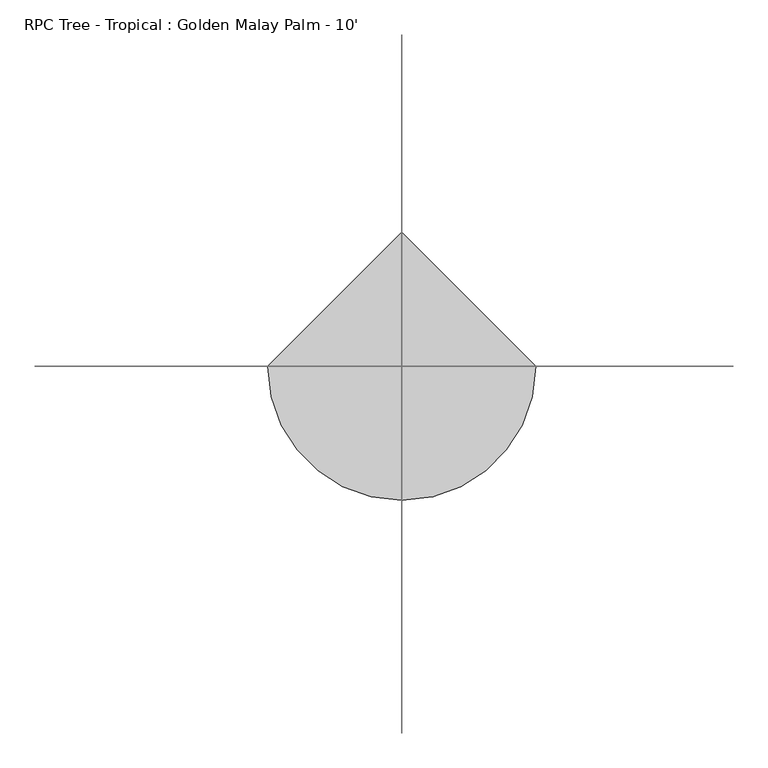
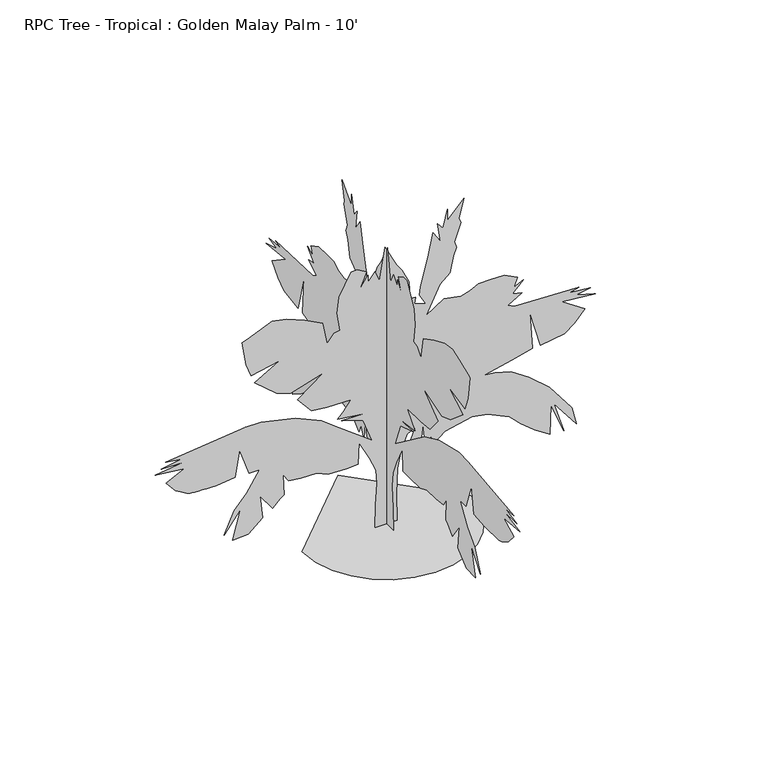
"""IFC4 building model written with IfcOpenShell, lengths in millimetres: geographic element geometry, RPC Tree - Tropical : Golden Malay Palm - 10'."""

from ifc_helpers import new_model, si_unit, origin, place, context, project, spatial, triangles, source, transform, mapped, element, save


def rpc_tree_tropical_golden_malay_palm_10_a310d7cf(model_context):
    return source(origin(), model_context, "Body", "Tessellation", [
        triangles([(9.89e-05, 133.5213922, 670.0644053), (0.0001158, 103.2936315, 529.0005229), (0.0001458, 93.2174569, 277.101182), (0.0001788, 98.2555397, 0.010878), (0.0001788, -113.3400931, 0.010878), (0.0001518, -108.30251, 226.7208087), (0.000126, -93.1884979, 443.3542972), (0.0001098, -103.2644181, 579.3813867), (9.23e-05, -163.7202029, 725.4820982), (6.95e-05, -264.479932, 916.9269533), (9.53e-05, -274.5561157, 700.292938), (9.59e-05, -385.3915197, 695.2536381), (9.53e-05, -561.7207641, 700.292938), (8.93e-05, -672.5587297, 750.671331), (8.93e-05, -828.7356068, 750.671331), (8.75e-05, -944.6103653, 765.7868328), (7.79e-05, -994.9887583, 846.3936859), (0.0001026, -984.9125565, 639.8358725), (0.0001056, -1025.2172184, 614.6467123), (0.0001146, -1095.7504858, 539.0766884), (9.47e-05, -1216.6620735, 705.3297672), (0.0001218, -1191.4703699, 478.6196228), (0.0001362, -1332.536832, 357.7080714), (0.0001368, -1483.6744091, 352.6712422), (0.0001026, -1403.067556, 639.8358725), (0.0001272, -1564.283733, 433.2780953), (0.000102, -1468.5613781, 644.8752451), (8.57e-05, -1347.6498631, 780.8998638), (6.23e-05, -1221.69883, 977.3814754), (6.23e-05, -1322.4607029, 977.3814754), (3.11e-05, -1413.1436852, 1239.3569092), (6.17e-05, -1458.4852489, 982.4207754), (6.41e-05, -1639.8538296, 962.2684444), (6.4e-05, -1687.1180958, 963.3555874), (6.38e-05, -1732.9753258, 964.4858963), (6.37e-05, -1776.0104897, 965.7050806), (6.35e-05, -1814.8165512, 967.0563789), (6.34e-05, -1847.9838581, 968.5828846), (6.32e-05, -1874.0976711, 970.3329231), (6.29e-05, -1891.7531342, 972.3446463), (6.24e-05, -1906.0304604, 976.2663546), (6.16e-05, -1922.6852577, 983.3606163), (6.04e-05, -1941.3262711, 993.0989754), (5.9e-05, -1961.5497459, 1004.9505775), (5.74e-05, -1982.9670433, 1018.3922716), (5.57e-05, -2005.1742634, 1032.8880438), (5.39e-05, -2027.7802963, 1047.9146702), (4.13e-05, -2118.4632786, 1153.7132269), (3.11e-05, -1947.1708271, 1239.3569092), (2.75e-05, -2224.261908, 1269.585442), (2.27e-05, -1952.2101997, 1309.8901039), (2.21e-05, -2168.844215, 1314.9270058), (1.79e-05, -1977.3993599, 1350.1949112), (1.55e-05, -2123.5001804, 1370.3471695), (5.3e-06, -1357.7259922, 1455.9909245), (5.3e-06, -1206.5858717, 1455.9909245), (1.43e-05, -874.0771706, 1380.4208279), (2.81e-05, -627.2171659, 1264.5486855), (4.37e-05, -455.9247508, 1133.5608959), (7.19e-05, -138.5302706, 896.7745497), (4.37e-05, -229.2143339, 1133.5608959), (3.59e-05, -435.7723835, 1199.0547907), (3.65e-05, -219.1381502, 1194.0154181), (3.23e-05, -471.0377455, 1229.2832508), (2.63e-05, -420.6568454, 1279.6617165), (1.43e-05, -340.0499923, 1380.4208279), (1.37e-05, -571.7995093, 1385.4602005), (1.19e-05, -722.9370501, 1400.5732315), (-7.4e-06, -858.9641396, 1561.7895538), (-2.96e-05, -607.064835, 1748.194891), (-1.82e-05, -924.4580343, 1652.4750069), (-2.36e-05, -1060.4851238, 1697.8165707), (-4.52e-05, -1272.0797665, 1879.1826805), (-6.14e-05, -1030.256591, 2015.2098427), (-5.48e-05, -1302.3082993, 1959.7921497), (-7.04e-05, -1352.6890903, 2090.7797939), (-9.86e-05, -1387.954525, 2327.5662128), (-9.98e-05, -1352.6890903, 2337.642342), (-0.000107, -1211.6227009, 2398.0967915), (-0.0001125, -1100.787315, 2443.4383553), (-0.0001095, -964.7627689, 2418.2491951), (-0.0001004, -788.4309448, 2342.6790985), (-8.96e-05, -617.1410368, 2251.9961163), (-6.32e-05, -571.7995093, 2030.3227283), (-7.28e-05, -506.3030711, 2110.9321976), (-7.4e-05, -445.848549, 2121.0083267), (-9.62e-05, -476.0770818, 2307.4138092), (-0.0001149, -455.9247508, 2463.5906136), (-0.0001401, -340.0499923, 2675.1776985), (-0.0001407, -284.6322812, 2680.2323318), (-0.0001347, -193.9479727, 2629.8386055), (-0.0001155, -259.443121, 2468.6301315), (-0.0001299, -178.834215, 2589.5288567), (-0.0001215, -178.834215, 2519.0084518), (-0.0001311, -113.3400931, 2599.6128342), (-0.0001185, -67.9985656, 2493.8192917), (-0.0001569, -17.6182708, 2816.2493202), (-0.0001311, 93.2174569, 2599.6128342), (-0.0001221, 148.6356586, 2524.0476791), (-0.0001052, 214.1292808, 2382.9839058), (-8.42e-05, 224.2057188, 2206.6545525), (-8.42e-05, 279.6234118, 2206.6545525), (-7.64e-05, 269.5472281, 2141.1607304), (-7.16e-05, 380.3826322, 2100.8560684), (-8.48e-05, 314.8887374, 2211.6914543), (-9.5e-05, 324.9649392, 2297.3376801), (-0.0001275, 395.4981703, 2569.3867722), (-0.0001551, 445.8764906, 2801.1362892), (-0.0001419, 516.4097217, 2690.2907295), (-0.0001641, 491.2205615, 2876.7011536), (-0.0001563, 541.5989182, 2811.219976), (-0.0001779, 586.9404093, 2992.5760574), (-0.0001641, 586.9404093, 2876.7011536), (-0.0001845, 743.1199024, 3047.9988373), (-0.0001623, 697.7783386, 2861.5881226), (-0.0001569, 712.8913696, 2816.2493202), (-0.0001359, 652.434304, 2639.922583), (-0.0001281, 672.586635, 2574.4158257), (-0.0001191, 642.3581022, 2498.8561935), (-9.98e-05, 607.0927766, 2337.642342), (-9.02e-05, 511.3703854, 2257.0328728), (-5.72e-05, 380.3826322, 1979.944408), (-7.1e-05, 551.6750836, 2095.8166958), (-6.68e-05, 712.8913696, 2060.5512611), (-6.98e-05, 803.5744246, 2085.7404213), (-7.52e-05, 884.1838211, 2131.0846012), (-7.52e-05, 995.019207, 2131.0846012), (-7.52e-05, 1131.0462965, 2131.0846012), (-6.74e-05, 1256.9946407, 2065.5906338), (-5.66e-05, 1226.7661079, 1974.9050354), (-6.2e-05, 1317.4517063, 2020.2465992), (-4.94e-05, 1211.6531496, 1914.4505859), (-4.7e-05, 1302.3362045, 1894.2981823), (-3.74e-05, 1166.3116585, 1813.6888584), (-3.32e-05, 1231.8054806, 1778.4234238), (-3.02e-05, 1851.4788483, 1753.2342636), (-2.78e-05, 1755.7564934, 1733.0820053), (-2.54e-05, 1962.3143795, 1712.9296017), (-2.24e-05, 1826.2896881, 1687.7404415), (-1.58e-05, 2007.655798, 1632.3227486), (-2e-05, 1685.2257694, 1667.5880379), (-1.9e-06, 1906.8966866, 1516.44799), (1.13e-05, 1806.1374298, 1405.6126041), (2.03e-05, 1710.4149296, 1330.0425076), (2.45e-05, 1478.6680286, 1294.7772182), (-1.94e-05, 1377.9063011, 1662.5486652), (2.45e-05, 1403.0979321, 1294.7772182), (3.05e-05, 1211.6531496, 1244.3962818), (3.77e-05, 934.5621414, 1183.9392162), (3.95e-05, 1040.3606981, 1168.8262579), (4.43e-05, 1196.5401913, 1128.5215233), (5.81e-05, 1367.8300266, 1012.6493082), (7.85e-05, 1564.3117836, 841.3568567), (0.0001128, 1780.9482697, 554.1896831), (0.0001338, 1826.2896881, 377.8604024), (0.0001007, 1609.6558182, 654.9514469), (0.0001374, 1705.3781731, 347.6318696), (0.0001014, 1579.4272854, 649.9120743), (0.0001356, 1569.3510109, 362.7474077), (0.0001242, 1423.2503357, 458.4697989), (0.0001116, 1292.2600754, 564.2658485), (9.83e-05, 1181.4246168, 675.1012344), (8.63e-05, 969.8300468, 775.8630346), (8.33e-05, 818.6899263, 801.0521948), (8.99e-05, 561.7512491, 745.6345018), (0.0001001, 455.9526924, 659.9882761), (9.05e-05, 425.7267031, 740.5976727), (0.0001032, 380.3826322, 634.7991159), (7.43e-05, 350.1566428, 876.6222187), (9.71e-05, 324.9649392, 685.1774363), (9.89e-05, 234.2813756, 670.0644053), (8.63e-05, 234.2813756, 775.8630346), (7.31e-05, 279.6234118, 886.6984205), (7.85e-05, 193.9774404, 841.3568567), (8.87e-05, 163.7496706, 755.710631), (133.5213922, 0.0001645, 670.0644053), (103.2936315, 0.0001813, 529.0005229), (93.2174569, 0.0002114, 277.101182), (98.2555397, 0.0002444, 0.0107758), (-113.3400931, 0.0002444, 0.0108645), (-108.30251, 0.0002174, 226.7208087), (-93.1887523, 0.0001915, 443.3542972), (-103.2644181, 0.0001753, 579.3813867), (-163.7204573, 0.0001579, 725.4820982), (-264.479932, 0.0001351, 916.9269533), (-274.5561157, 0.0001609, 700.292938), (-385.3915197, 0.0001615, 695.2536381), (-561.7233075, 0.0001609, 700.292938), (-672.5587297, 0.0001549, 750.671331), (-828.7356068, 0.0001549, 750.671331), (-944.6103653, 0.0001531, 765.7868328), (-994.9912291, 0.0001435, 846.3936859), (-984.9125565, 0.0001681, 639.8358725), (-1025.2172184, 0.0001711, 614.6467123), (-1095.7504858, 0.0001801, 539.0766884), (-1216.6620735, 0.0001603, 705.3297672), (-1191.4703699, 0.0001873, 478.6196228), (-1332.536832, 0.0002018, 357.7080714), (-1483.6744091, 0.0002024, 352.6712422), (-1403.067556, 0.0001681, 639.8358725), (-1564.283733, 0.0001927, 433.2780953), (-1468.5613781, 0.0001675, 644.8752451), (-1347.6498631, 0.0001513, 780.8998638), (-1221.69883, 0.0001279, 977.3814754), (-1322.4607029, 0.0001279, 977.3814754), (-1413.1436852, 9.67e-05, 1239.3569092), (-1458.4852489, 0.0001273, 982.4207754), (-1639.8538296, 0.0001297, 962.2684444), (-1687.1180958, 0.0001296, 963.3555874), (-1732.9753258, 0.0001294, 964.4858963), (-1776.0104897, 0.0001293, 965.7050806), (-1814.8165512, 0.0001291, 967.0563789), (-1847.9838581, 0.0001289, 968.5828846), (-1874.0976711, 0.0001287, 970.3329231), (-1891.7531342, 0.0001285, 972.3446463), (-1906.0304604, 0.000128, 976.2663546), (-1922.6852577, 0.0001272, 983.3606163), (-1941.3262711, 0.000126, 993.0989754), (-1961.5497459, 0.0001246, 1004.9505775), (-1982.9670433, 0.000123, 1018.3922716), (-2005.1742634, 0.0001213, 1032.8880438), (-2027.7802963, 0.0001195, 1047.9146702), (-2118.4632786, 0.0001069, 1153.7132269), (-1947.1708271, 9.67e-05, 1239.3569092), (-2224.261908, 9.31e-05, 1269.585442), (-1952.2101997, 8.82e-05, 1309.8901039), (-2168.844215, 8.76e-05, 1314.9270058), (-1977.3993599, 8.34e-05, 1350.1949112), (-2123.5001804, 8.1e-05, 1370.3471695), (-1357.7259922, 7.08e-05, 1455.9909245), (-1206.5858717, 7.08e-05, 1455.9909245), (-874.0771706, 7.98e-05, 1380.4208279), (-627.2171659, 9.37e-05, 1264.5486855), (-455.9247508, 0.0001093, 1133.5608959), (-138.5302706, 0.0001375, 896.7745497), (-229.2145882, 0.0001093, 1133.5608959), (-435.7723835, 0.0001015, 1199.0547907), (-219.1381502, 0.0001021, 1194.0154181), (-471.0377455, 9.79e-05, 1229.2832508), (-420.6593888, 9.18e-05, 1279.6617165), (-340.0499923, 7.98e-05, 1380.4208279), (-571.7995093, 7.92e-05, 1385.4602005), (-722.9370501, 7.74e-05, 1400.5732315), (-858.9641396, 5.82e-05, 1561.7895538), (-607.064835, 3.6e-05, 1748.194891), (-924.4580343, 4.74e-05, 1652.4750069), (-1060.4851238, 4.2e-05, 1697.8165707), (-1272.0797665, 2.04e-05, 1879.1826805), (-1030.256591, 4.2e-06, 2015.2098427), (-1302.3082993, 1.08e-05, 1959.7921497), (-1352.6890903, -4.8e-06, 2090.7797939), (-1387.954525, -3.31e-05, 2327.5662128), (-1352.6890903, -3.43e-05, 2337.642342), (-1211.6227009, -4.15e-05, 2398.0967915), (-1100.787315, -4.69e-05, 2443.4383553), (-964.7627689, -4.39e-05, 2418.2491951), (-788.4309448, -3.49e-05, 2342.6790985), (-617.1410368, -2.41e-05, 2251.9961163), (-571.7995093, 2.4e-06, 2030.3227283), (-506.3030711, -7.2e-06, 2110.9321976), (-445.848549, -8.4e-06, 2121.0083267), (-476.0770818, -3.07e-05, 2307.4138092), (-455.9247508, -4.93e-05, 2463.5906136), (-340.0499923, -7.45e-05, 2675.1776985), (-284.6322812, -7.51e-05, 2680.2323318), (-193.948227, -6.91e-05, 2629.8386055), (-259.443121, -4.99e-05, 2468.6301315), (-178.834215, -6.43e-05, 2589.5288567), (-178.834215, -5.59e-05, 2519.0084518), (-113.3400931, -6.55e-05, 2599.6128342), (-67.9985656, -5.29e-05, 2493.8192917), (-17.6183468, -9.13e-05, 2816.2493202), (93.2174569, -6.55e-05, 2599.6128342), (148.6356586, -5.65e-05, 2524.0476791), (214.1292808, -3.97e-05, 2382.9839058), (224.2054645, -1.87e-05, 2206.6545525), (279.6234118, -1.87e-05, 2206.6545525), (269.5472281, -1.08e-05, 2141.1607304), (380.3826322, -6e-06, 2100.8560684), (314.8887374, -1.93e-05, 2211.6914543), (324.9649392, -2.95e-05, 2297.3376801), (395.4981703, -6.19e-05, 2569.3867722), (445.8764906, -8.95e-05, 2801.1362892), (516.4097217, -7.63e-05, 2690.2907295), (491.2205615, -9.85e-05, 2876.7011536), (541.5989182, -9.07e-05, 2811.219976), (586.9404093, -0.0001123, 2992.5760574), (586.9404093, -9.85e-05, 2876.7011536), (743.1199024, -0.000119, 3047.9988373), (697.7757952, -9.67e-05, 2861.5881226), (712.8913696, -9.13e-05, 2816.2493202), (652.434304, -7.03e-05, 2639.922583), (672.586635, -6.25e-05, 2574.4158257), (642.3581022, -5.35e-05, 2498.8561935), (607.0927766, -3.43e-05, 2337.642342), (511.3703854, -2.47e-05, 2257.0328728), (380.3826322, 8.4e-06, 1979.944408), (551.6750836, -5.4e-06, 2095.8166958), (712.8913696, -1.2e-06, 2060.5512611), (803.5744246, -4.2e-06, 2085.7404213), (884.1838211, -9.6e-06, 2131.0846012), (995.019207, -9.6e-06, 2131.0846012), (1131.0462965, -9.6e-06, 2131.0846012), (1256.9946407, -1.8e-06, 2065.5906338), (1226.7661079, 9e-06, 1974.9050354), (1317.4517063, 3.6e-06, 2020.2465992), (1211.6531496, 1.62e-05, 1914.4505859), (1302.3362045, 1.86e-05, 1894.2981823), (1166.3116585, 2.82e-05, 1813.6888584), (1231.8054806, 3.24e-05, 1778.4234238), (1851.4788483, 3.54e-05, 1753.2342636), (1755.7564934, 3.78e-05, 1733.0820053), (1962.3143795, 4.02e-05, 1712.9296017), (1826.2896881, 4.32e-05, 1687.7404415), (2007.655798, 4.98e-05, 1632.3227486), (1685.2232986, 4.56e-05, 1667.5880379), (1906.8966866, 6.36e-05, 1516.44799), (1806.1374298, 7.68e-05, 1405.6126041), (1710.4149296, 8.58e-05, 1330.0425076), (1478.6680286, 9e-05, 1294.7772182), (1377.9063011, 4.62e-05, 1662.5486652), (1403.0954613, 9e-05, 1294.7772182), (1211.6531496, 9.61e-05, 1244.3962818), (934.5621414, 0.0001033, 1183.9392162), (1040.3606981, 0.0001051, 1168.8262579), (1196.5401913, 0.0001099, 1128.5215233), (1367.8300266, 0.0001237, 1012.6493082), (1564.3117836, 0.0001441, 841.3568567), (1780.9456535, 0.0001783, 554.1896831), (1826.2896881, 0.0001994, 377.8604024), (1609.6558182, 0.0001663, 654.9514469), (1705.3757023, 0.000203, 347.6318696), (1579.4272854, 0.0001669, 649.9120743), (1569.3510109, 0.0002012, 362.7474077), (1423.2503357, 0.0001897, 458.4672918), (1292.2600754, 0.0001771, 564.2658485), (1181.4246168, 0.0001639, 675.1012344), (969.8300468, 0.0001519, 775.8630346), (818.6899263, 0.0001489, 801.0521948), (561.7512491, 0.0001555, 745.6345018), (455.9526924, 0.0001657, 659.9882761), (425.7241596, 0.0001561, 740.5951292), (380.3826322, 0.0001687, 634.7991159), (350.1566428, 0.0001399, 876.6222187), (324.9649392, 0.0001627, 685.1774363), (234.2813756, 0.0001645, 670.0644053), (234.2813756, 0.0001519, 775.8630346), (279.6234118, 0.0001387, 886.6984205), (193.9774404, 0.0001441, 841.3568567), (163.7496706, 0.0001543, 755.710631), (-812.451717, 0.0, 7.05e-05), (-790.9734495, -186.160076, 7.3e-05), (-729.802692, -357.1187905, 8.03e-05), (-633.8364567, -507.9769515, 9.18e-05), (-507.9769515, -633.8364567, 0.0001068), (-357.1187905, -729.802692, 1.08e-05), (-186.1598216, -790.9734495, 3.12e-05), (3.55e-05, -812.451717, 5.34e-05), (186.160076, -790.9734495, 7.56e-05), (357.1187905, -729.802692, 9.6e-05), (507.9769515, -633.8364567, 0.0), (633.8364567, -507.9769515, 1.5e-05), (729.802692, -357.1187905, 2.64e-05), (790.9734495, -186.1598216, 3.37e-05), (812.451717, 7.1e-05, 3.63e-05), (-0.0001065, 812.451717, 5.34e-05)], [[157, 156, 158], [140, 139, 141], [52, 51, 53], [26, 25, 27], [112, 111, 113], [136, 135, 137], [54, 53, 55], [50, 49, 51], [138, 137, 139], [62, 61, 63], [131, 130, 132], [155, 154, 156], [154, 153, 156], [114, 113, 115], [110, 109, 111], [168, 167, 169], [93, 92, 94], [97, 96, 98], [139, 137, 141], [133, 132, 134], [108, 107, 109], [137, 135, 141], [27, 25, 28], [64, 63, 65], [159, 158, 160], [95, 94, 96], [53, 51, 55], [73, 72, 74], [166, 165, 167], [24, 23, 25], [23, 22, 25], [22, 21, 25], [25, 21, 28], [65, 63, 66], [48, 47, 49], [20, 19, 21], [171, 170, 172], [170, 169, 172], [172, 169, 173], [102, 101, 103], [142, 141, 143], [156, 153, 158], [69, 68, 70], [68, 67, 70], [28, 21, 29], [5, 4, 6], [4, 3, 6], [6, 3, 7], [3, 2, 7], [7, 2, 8], [2, 1, 8], [160, 158, 161], [8, 1, 9], [98, 96, 99], [11, 10, 12], [145, 144, 146], [144, 143, 146], [143, 141, 146], [141, 135, 146], [67, 66, 70], [91, 90, 92], [90, 89, 92], [89, 88, 92], [77, 76, 78], [88, 87, 92], [1, 175, 9], [129, 128, 130], [75, 74, 76], [51, 49, 55], [47, 46, 49], [147, 146, 148], [158, 153, 161], [153, 152, 161], [161, 152, 162], [162, 152, 163], [152, 151, 163], [151, 150, 163], [150, 149, 163], [163, 149, 164], [72, 71, 74], [71, 70, 74], [76, 74, 78], [78, 74, 79], [79, 74, 80], [80, 74, 81], [81, 74, 82], [74, 70, 82], [82, 70, 83], [83, 70, 84], [32, 31, 33], [146, 135, 148], [148, 135, 149], [135, 134, 149], [99, 96, 100], [46, 45, 49], [30, 29, 31], [9, 175, 10], [175, 174, 10], [45, 44, 49], [49, 44, 55], [44, 43, 55], [43, 42, 55], [42, 41, 55], [41, 40, 55], [40, 39, 55], [39, 38, 55], [38, 37, 55], [37, 36, 55], [36, 35, 55], [35, 34, 55], [34, 33, 55], [33, 31, 55], [55, 31, 56], [31, 29, 56], [56, 29, 57], [57, 29, 58], [100, 96, 101], [29, 21, 58], [115, 113, 116], [116, 113, 117], [113, 111, 117], [111, 109, 117], [109, 107, 117], [117, 107, 118], [118, 107, 119], [107, 106, 119], [119, 106, 120], [120, 106, 121], [106, 105, 121], [105, 104, 121], [121, 104, 122], [104, 103, 122], [167, 165, 169], [12, 10, 13], [87, 86, 92], [164, 149, 165], [165, 149, 169], [18, 17, 19], [19, 17, 21], [21, 17, 58], [58, 17, 59], [17, 16, 59], [16, 15, 59], [15, 14, 59], [14, 13, 59], [13, 10, 59], [59, 10, 60], [10, 174, 60], [60, 174, 61], [61, 174, 63], [174, 173, 63], [128, 127, 130], [130, 127, 132], [132, 127, 134], [127, 126, 134], [126, 125, 134], [134, 125, 149], [125, 124, 149], [149, 124, 169], [124, 123, 169], [123, 122, 169], [169, 122, 173], [173, 122, 63], [63, 122, 66], [66, 122, 70], [122, 103, 70], [70, 103, 84], [84, 103, 85], [85, 103, 86], [103, 101, 86], [101, 96, 86], [86, 96, 92], [96, 94, 92], [331, 332, 333], [314, 315, 316], [226, 227, 228], [200, 201, 202], [286, 287, 288], [310, 311, 312], [228, 229, 230], [224, 225, 226], [312, 313, 314], [236, 237, 238], [305, 306, 307], [329, 330, 331], [328, 329, 331], [288, 289, 290], [284, 285, 286], [342, 343, 344], [267, 268, 269], [271, 272, 273], [312, 314, 316], [307, 308, 309], [282, 283, 284], [310, 312, 316], [200, 202, 203], [238, 239, 240], [333, 334, 335], [269, 270, 271], [226, 228, 230], [247, 248, 249], [340, 341, 342], [198, 199, 200], [197, 198, 200], [196, 197, 200], [196, 200, 203], [238, 240, 241], [222, 223, 224], [194, 195, 196], [345, 346, 347], [344, 345, 347], [344, 347, 348], [276, 277, 278], [316, 317, 318], [328, 331, 333], [243, 244, 245], [242, 243, 245], [196, 203, 204], [179, 180, 181], [178, 179, 181], [178, 181, 182], [177, 178, 182], [177, 182, 183], [176, 177, 183], [333, 335, 336], [176, 183, 184], [271, 273, 274], [185, 186, 187], [319, 320, 321], [318, 319, 321], [316, 318, 321], [310, 316, 321], [241, 242, 245], [265, 266, 267], [264, 265, 267], [263, 264, 267], [251, 252, 253], [262, 263, 267], [350, 176, 184], [303, 304, 305], [249, 250, 251], [224, 226, 230], [221, 222, 224], [321, 322, 323], [328, 333, 336], [327, 328, 336], [327, 336, 337], [327, 337, 338], [326, 327, 338], [325, 326, 338], [324, 325, 338], [324, 338, 339], [246, 247, 249], [245, 246, 249], [249, 251, 253], [249, 253, 254], [249, 254, 255], [249, 255, 256], [249, 256, 257], [245, 249, 257], [245, 257, 258], [245, 258, 259], [206, 207, 208], [310, 321, 323], [310, 323, 324], [309, 310, 324], [271, 274, 275], [220, 221, 224], [204, 205, 206], [350, 184, 185], [349, 350, 185], [219, 220, 224], [219, 224, 230], [218, 219, 230], [217, 218, 230], [216, 217, 230], [215, 216, 230], [214, 215, 230], [213, 214, 230], [212, 213, 230], [211, 212, 230], [210, 211, 230], [209, 210, 230], [208, 209, 230], [206, 208, 230], [206, 230, 231], [204, 206, 231], [204, 231, 232], [204, 232, 233], [271, 275, 276], [196, 204, 233], [288, 290, 291], [288, 291, 292], [286, 288, 292], [284, 286, 292], [282, 284, 292], [282, 292, 293], [282, 293, 294], [281, 282, 294], [281, 294, 295], [281, 295, 296], [280, 281, 296], [279, 280, 296], [279, 296, 297], [278, 279, 297], [340, 342, 344], [185, 187, 188], [261, 262, 267], [324, 339, 340], [324, 340, 344], [192, 193, 194], [192, 194, 196], [192, 196, 233], [192, 233, 234], [191, 192, 234], [190, 191, 234], [189, 190, 234], [188, 189, 234], [185, 188, 234], [185, 234, 235], [349, 185, 235], [349, 235, 236], [349, 236, 238], [348, 349, 238], [302, 303, 305], [302, 305, 307], [302, 307, 309], [301, 302, 309], [300, 301, 309], [300, 309, 324], [299, 300, 324], [299, 324, 344], [298, 299, 344], [297, 298, 344], [297, 344, 348], [297, 348, 238], [297, 238, 241], [297, 241, 245], [278, 297, 245], [278, 245, 259], [278, 259, 260], [278, 260, 261], [276, 278, 261], [271, 276, 261], [271, 261, 267], [269, 271, 267], [365, 366, 351], [364, 365, 351], [364, 351, 352], [363, 364, 352], [363, 352, 353], [363, 353, 354], [362, 363, 354], [361, 362, 354], [361, 354, 355], [361, 355, 356], [361, 356, 357], [361, 357, 358], [361, 358, 359], [361, 359, 360]], closed=False),
    ])


if __name__ == "__main__":
    model = new_model("IFC4")
    model_context = context("Model", 3, world=origin())
    ifc_project = project(units=[si_unit("LENGTHUNIT", "METRE", prefix="MILLI")], contexts=[model_context])
    site = spatial("IfcSite", under=ifc_project)
    building = spatial("IfcBuilding", under=site)
    placement = place(None, origin())
    rpc_tree_tropical_golden_malay_palm_10_shape = rpc_tree_tropical_golden_malay_palm_10_a310d7cf(model_context)
    element("IfcGeographicElement", 1, ObjectType="RPC Tree - Tropical : Golden Malay Palm - 10'", at=placement, inside=building, context=model_context, shape_type="MappedRepresentation", body=[
        mapped(rpc_tree_tropical_golden_malay_palm_10_shape, transform((0.0, 0.0, 0.0), x_axis=(1.0, 0.0, 0.0), y_axis=(0.0, 1.0, 0.0), z_axis=(0.0, 0.0, 1.0))),
    ])
    save(model, "model.ifc")

# Revit data of these elements
# Type "RPC Tree - Tropical : Golden Malay Palm - 10'"
#   built-in parameter 1005198 = "{2, 15},{39, RPC-16-FXGM-2RXX-PGXL-E000-ST1L-LVER-AU},{1, 0},{1, 0},{2, 13},{1, 8},{5, Color},{1, 0},{1, 0},{3, 0.8},{3, 0.8},{3, 0.8},{1, 8},{7, BBoxMin},{1, 0},{1, 0},{1, 0},{1, 0},{1, 0},{1, 8},{7, BBoxMax},{1, 0},{1, 0},{1, 0},{1, 0},{1, 0},{2, 11},{9, RPCTypeId},{1, 0},{1, 0},{39, RPC-16-FXGM-2RXX-PGXL-E000-ST1L-LVER-AU},{1, 6},{14, RPCPlantHeight},{1, 0},{1, 0},{2, 10},{2, 11},{7, keyword},{1, 0},{1, 0},{35, :RPCs:Trees [Tropical]:Geometry:RPC},{2, 11},{8, category},{1, 0},{1, 0},{16, Trees [Tropical]},{2, 11},{12, LocalizedUID},{1, 0},{1, 0},{17, Golden Malay Palm},{2, 14},{6, Height},{1, 0},{1, 0},{2, 10},{1, 2},{16, Cast Reflections},{1, 0},{1, 0},{1, 0},{1, 2},{12, Cast Shadows},{1, 0},{1, 0},{1, 1},{1, 2},{9, Lock View},{1, 0},{1, 0},{1, 0},{1, 4},{5, ViewC},{1, 0},{1, 0},{1, 0},{21, assetlibrary_base.fbx},{1, 5},"
#   built-in parameter 1005195 = "RPC-16-FXGM-2RXX-PGXL-E000-ST1L-LVER-AU"
#   Type Comments = "Golden Malay Palm"
#   Assembly Code = "G2050500"
#   Height = 10' - 0"
#   Plan Symbol = element 361270
#   Default Elevation = 0
